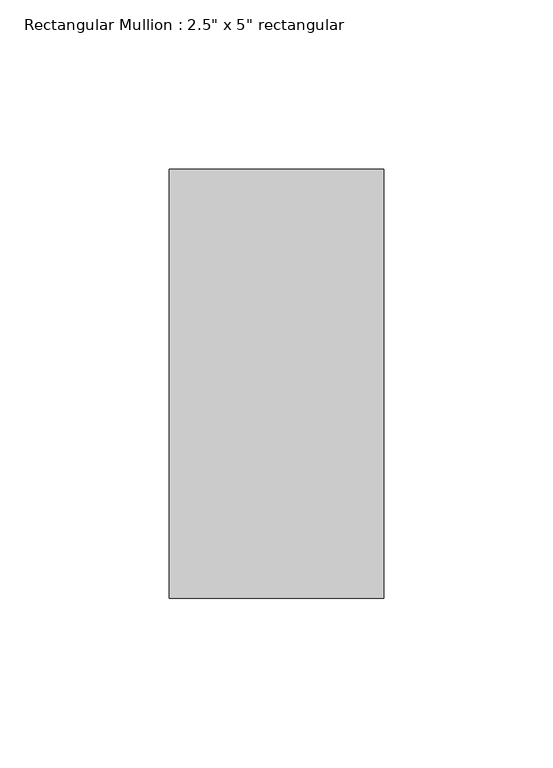
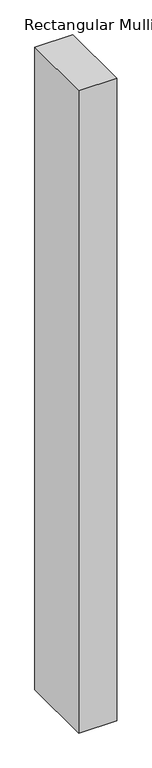
"""IFC4 building model written with IfcOpenShell, lengths in millimetres: member geometry."""

from ifc_helpers import new_model, si_unit, frame, origin, place, context, project, spatial, polyline, outline, extrude, source, transform, mapped, element, save


def member_54a35e60(model_context):
    return source(origin(), model_context, "Body", "SweptSolid", [
        extrude(outline(polyline([(0.0, 63.5), (0.0, -63.5), (-63.5, -63.5), (-63.5, 63.5), (0.0, 63.5)])), frame((0.0, 0.0, -1136.65), z_axis=(0.0, 0.0, 1.0), x_axis=(1.0, 0.0, 0.0)), (0.0, 0.0, 1.0), 1136.65),
    ])


if __name__ == "__main__":
    model = new_model("IFC4")
    model_context = context("Model", 3, world=origin())
    ifc_project = project(units=[si_unit("LENGTHUNIT", "METRE", prefix="MILLI")], contexts=[model_context])
    site = spatial("IfcSite", under=ifc_project)
    building = spatial("IfcBuilding", under=site)
    placement = place(None, origin())
    member_shape = member_54a35e60(model_context)
    element("IfcMember", 1, ObjectType="Rectangular Mullion : 2.5\" x 5\" rectangular", at=placement, inside=building, context=model_context, shape_type="MappedRepresentation", body=[
        mapped(member_shape, transform((0.0, 0.0, 0.0), x_axis=(1.0, 0.0, 0.0), y_axis=(0.0, 1.0, 0.0), z_axis=(0.0, 0.0, 1.0))),
    ])
    save(model, "model.ifc")

# Revit data of these elements
# Type "Rectangular Mullion : 2.5\" x 5\" rectangular"
#   built-in parameter 1007304 = 0.416667 (stored number, unit not read)
#   built-in parameter 1007301 = 0.104167 (stored number, unit not read)
#   built-in parameter 1007300 = 0.104167 (stored number, unit not read)
# Element 1 (IfcMember, "Rectangular Mullion : 2.5\" x 5\" rectangular")
#   Materials on its faces: "Aluminum"
# Materials
#   "Aluminum": class "Metal", colour RGB 247 247 247, transparency 0, Description = "Aluminum 6061", Cost = 0
